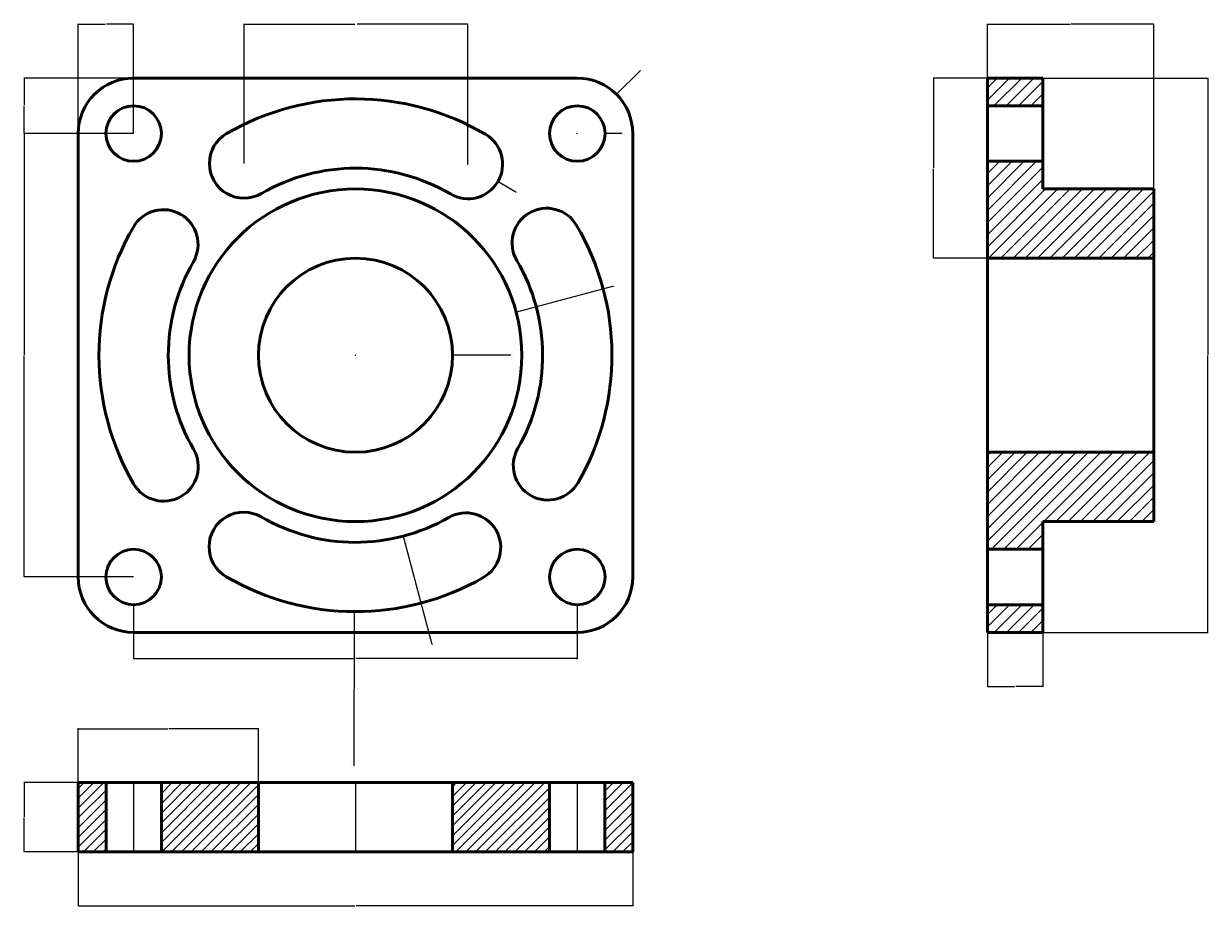
# Model space of a CAD drawing. Units: inches. Extents: x 17 to 444, y -186 to 133.
import ezdxf

# ---------------------------------------------------------------- set-up
doc = ezdxf.new("R2010")
doc.units = ezdxf.units.IN
doc.header["$MEASUREMENT"] = 0
doc.linetypes.add('CENTER', pattern=[50.8, 31.75, -6.35, 6.35, -6.35])
for name, color, linetype, lineweight in [('M-CNTR', 4, 'CENTER', 18), ('M-DIMS', 2, 'Continuous', 18), ('M-HATC', 8, 'Continuous', 18), ('M-OUTL', 7, 'Continuous', 50)]:
    doc.layers.add(name, color=color, linetype=linetype, lineweight=lineweight)
doc.styles.get("Standard").update_dxf_attribs({"font": 'arial.ttf'})
doc.dimstyles.get("Standard").update_dxf_attribs({"dimtxt": 0.18, "dimasz": 0.18, "dimexe": 0.18, "dimexo": 0.0625, "dimgap": 0.09, "dimtad": 0, "dimtih": 1, "dimtoh": 1, "dimdec": 4, "dimzin": 0, "dimdsep": 46, "dimtxsty": 'Standard', "dimcen": 0.09, "dimadec": 0, "dimazin": 0, "dimtfac": 1, "dimtdec": 4, "dimtofl": 0, "dimtmove": 0, "dimatfit": 3, "dimfxl": 1, "dimtolj": 1, "dimtzin": 0, "dimarcsym": 0})
pattern_1 = [(45, (-581.398, -124.7495), (-2.209709, 2.209709), [])]
pattern_2 = [(45, (-581.398, -124.7495), (-1.767767, 1.767767), [])]

# ---------------------------------------------------------------- blocks, each defined once
blk = doc.blocks.new('FLANGE-MOUNT-HOLE-D20')
blk.add_circle((10, 10), 10)
blk = doc.blocks.new('*D2')
at = {"layer": 'Defpoints', "color": 0, "transparency": 16777216}
for p in [(36.63, -165.99), (236.63, -165.99), (236.63, -185.44)]:
    blk.add_point(p, dxfattribs=at)
at = {"layer": 'M-DIMS', "color": 0, "lineweight": -2, "transparency": 16777216}
for p, q in [((36.63, -166.06), (36.63, -185.62)), ((236.63, -166.06), (236.63, -185.62)), ((36.81, -185.44), (136.34, -185.44)), ((236.45, -185.44), (136.92, -185.44))]:
    blk.add_line(p, q, dxfattribs=at)
at = {"layer": 'M-DIMS', "color": 0, "transparency": 16777216}
for points in [[(36.81, -185.41), (36.81, -185.47), (36.63, -185.44)], [(236.45, -185.41), (236.45, -185.47), (236.63, -185.44)]]:
    blk.add_solid(points, dxfattribs=at)
at = {"layer": 'M-DIMS', "color": 0, "transparency": 16777216, "insert": (136.63, -185.44), "char_height": 0.18, "attachment_point": 5}
blk.add_mtext('\\A1;200', dxfattribs=at)
blk = doc.blocks.new('*D3')
at = {"layer": 'Defpoints', "color": 0, "transparency": 16777216}
for p in [(384.54, 113.19), (443.99, 113.19), (384.54, -86.81)]:
    blk.add_point(p, dxfattribs=at)
at = {"layer": 'M-DIMS', "color": 0, "lineweight": -2, "transparency": 16777216}
for p, q in [((384.6, 113.19), (444.17, 113.19)), ((443.99, 113.01), (443.99, 13.37)), ((443.99, -86.63), (443.99, 13.01)), ((384.6, -86.81), (444.17, -86.81))]:
    blk.add_line(p, q, dxfattribs=at)
at = {"layer": 'M-DIMS', "color": 0, "transparency": 16777216}
for points in [[(443.96, 113.01), (444.02, 113.01), (443.99, 113.19)], [(443.96, -86.63), (444.02, -86.63), (443.99, -86.81)]]:
    blk.add_solid(points, dxfattribs=at)
at = {"layer": 'M-DIMS', "color": 0, "transparency": 16777216, "insert": (443.99, 13.19), "char_height": 0.18, "attachment_point": 5}
blk.add_mtext('\\A1;200', dxfattribs=at)
blk = doc.blocks.new('*D4')
at = {"layer": 'Defpoints', "color": 0, "transparency": 16777216}
for p in [(56.63, -76.81), (216.63, -76.81), (56.63, -96.26)]:
    blk.add_point(p, dxfattribs=at)
at = {"layer": 'M-DIMS', "color": 0, "lineweight": -2, "transparency": 16777216}
for p, q in [((56.63, -76.87), (56.63, -96.44)), ((216.63, -76.87), (216.63, -96.44)), ((56.81, -96.26), (136.35, -96.26)), ((216.45, -96.26), (136.91, -96.26))]:
    blk.add_line(p, q, dxfattribs=at)
at = {"layer": 'M-DIMS', "color": 0, "transparency": 16777216}
for points in [[(56.81, -96.23), (56.81, -96.29), (56.63, -96.26)], [(216.45, -96.23), (216.45, -96.29), (216.63, -96.26)]]:
    blk.add_solid(points, dxfattribs=at)
at = {"layer": 'M-DIMS', "color": 0, "transparency": 16777216, "insert": (136.63, -96.26), "char_height": 0.18, "attachment_point": 5}
blk.add_mtext('\\A1;160', dxfattribs=at)
blk = doc.blocks.new('*D5')
at = {"layer": 'Defpoints', "color": 0, "transparency": 16777216}
for p in [(17.18, 93.19), (56.63, 93.19), (56.63, -66.81)]:
    blk.add_point(p, dxfattribs=at)
at = {"layer": 'M-DIMS', "color": 0, "lineweight": -2, "transparency": 16777216}
for p, q in [((56.56, 93.19), (17, 93.19)), ((17.18, 93.01), (17.18, 13.37)), ((17.18, -66.63), (17.18, 13.01)), ((56.56, -66.81), (17, -66.81))]:
    blk.add_line(p, q, dxfattribs=at)
at = {"layer": 'M-DIMS', "color": 0, "transparency": 16777216}
for points in [[(17.15, 93.01), (17.21, 93.01), (17.18, 93.19)], [(17.15, -66.63), (17.21, -66.63), (17.18, -66.81)]]:
    blk.add_solid(points, dxfattribs=at)
at = {"layer": 'M-DIMS', "color": 0, "transparency": 16777216, "insert": (17.18, 13.19), "char_height": 0.18, "attachment_point": 5}
blk.add_mtext('\\A1;160', dxfattribs=at)
blk = doc.blocks.new('*D6')
at = {"layer": 'Defpoints', "color": 0, "transparency": 16777216}
for p in [(56.63, 132.64), (36.63, 93.19), (56.63, 93.19)]:
    blk.add_point(p, dxfattribs=at)
at = {"layer": 'M-DIMS', "color": 0, "lineweight": -2, "transparency": 16777216}
for p, q in [((36.63, 93.25), (36.63, 132.82)), ((36.81, 132.64), (46.41, 132.64)), ((56.45, 132.64), (46.85, 132.64)), ((56.63, 93.25), (56.63, 132.82))]:
    blk.add_line(p, q, dxfattribs=at)
at = {"layer": 'M-DIMS', "color": 0, "transparency": 16777216}
for points in [[(36.81, 132.67), (36.81, 132.61), (36.63, 132.64)], [(56.45, 132.67), (56.45, 132.61), (56.63, 132.64)]]:
    blk.add_solid(points, dxfattribs=at)
at = {"layer": 'M-DIMS', "color": 0, "transparency": 16777216, "insert": (46.63, 132.64), "char_height": 0.18, "attachment_point": 5}
blk.add_mtext('\\A1;20', dxfattribs=at)
blk = doc.blocks.new('*D7')
at = {"layer": 'Defpoints', "color": 0, "transparency": 16777216}
for p in [(17.18, 113.19), (56.63, 113.19), (56.63, 93.19)]:
    blk.add_point(p, dxfattribs=at)
at = {"layer": 'M-DIMS', "color": 0, "lineweight": -2, "transparency": 16777216}
for p, q in [((56.56, 113.19), (17, 113.19)), ((17.18, 113.01), (17.18, 103.37)), ((17.18, 93.37), (17.18, 103.01)), ((56.56, 93.19), (17, 93.19))]:
    blk.add_line(p, q, dxfattribs=at)
at = {"layer": 'M-DIMS', "color": 0, "transparency": 16777216}
for points in [[(17.15, 113.01), (17.21, 113.01), (17.18, 113.19)], [(17.15, 93.37), (17.21, 93.37), (17.18, 93.19)]]:
    blk.add_solid(points, dxfattribs=at)
at = {"layer": 'M-DIMS', "color": 0, "transparency": 16777216, "insert": (17.18, 103.19), "char_height": 0.18, "attachment_point": 5}
blk.add_mtext('\\A1;20', dxfattribs=at)
blk = doc.blocks.new('*D8')
at = {"layer": 'Defpoints', "color": 0, "transparency": 16777216}
for p in [(177.18, 132.64), (96.44, 82.37), (177.18, 82.15)]:
    blk.add_point(p, dxfattribs=at)
at = {"layer": 'M-DIMS', "color": 0, "lineweight": -2, "transparency": 16777216}
for p, q in [((96.44, 82.43), (96.44, 132.82)), ((96.62, 132.64), (136.42, 132.64)), ((177, 132.64), (137.21, 132.64)), ((177.18, 82.21), (177.18, 132.82))]:
    blk.add_line(p, q, dxfattribs=at)
at = {"layer": 'M-DIMS', "color": 0, "transparency": 16777216}
for points in [[(96.62, 132.67), (96.62, 132.61), (96.44, 132.64)], [(177, 132.67), (177, 132.61), (177.18, 132.64)]]:
    blk.add_solid(points, dxfattribs=at)
at = {"layer": 'M-DIMS', "color": 0, "transparency": 16777216, "insert": (136.81, 132.64), "char_height": 0.18, "attachment_point": 5}
blk.add_mtext('\\A1;80.74', dxfattribs=at)
blk = doc.blocks.new('*D9')
at = {"layer": 'Defpoints', "color": 0, "transparency": 16777216}
for p in [(364.54, -86.81), (384.54, -86.81), (364.54, -106.26)]:
    blk.add_point(p, dxfattribs=at)
at = {"layer": 'M-DIMS', "color": 0, "lineweight": -2, "transparency": 16777216}
for p, q in [((364.54, -86.87), (364.54, -106.44)), ((384.54, -86.87), (384.54, -106.44)), ((364.72, -106.26), (374.32, -106.26)), ((384.36, -106.26), (374.76, -106.26))]:
    blk.add_line(p, q, dxfattribs=at)
at = {"layer": 'M-DIMS', "color": 0, "transparency": 16777216}
for points in [[(364.72, -106.23), (364.72, -106.29), (364.54, -106.26)], [(384.36, -106.23), (384.36, -106.29), (384.54, -106.26)]]:
    blk.add_solid(points, dxfattribs=at)
at = {"layer": 'M-DIMS', "color": 0, "transparency": 16777216, "insert": (374.54, -106.26), "char_height": 0.18, "attachment_point": 5}
blk.add_mtext('\\A1;20', dxfattribs=at)
blk = doc.blocks.new('*D10')
at = {"layer": 'Defpoints', "color": 0, "transparency": 16777216}
for p in [(424.54, 132.64), (364.54, 113.19), (424.54, 73.19)]:
    blk.add_point(p, dxfattribs=at)
at = {"layer": 'M-DIMS', "color": 0, "lineweight": -2, "transparency": 16777216}
for p, q in [((364.54, 113.25), (364.54, 132.82)), ((364.72, 132.64), (394.32, 132.64)), ((424.36, 132.64), (394.76, 132.64)), ((424.54, 73.25), (424.54, 132.82))]:
    blk.add_line(p, q, dxfattribs=at)
at = {"layer": 'M-DIMS', "color": 0, "transparency": 16777216}
for points in [[(364.72, 132.67), (364.72, 132.61), (364.54, 132.64)], [(424.36, 132.67), (424.36, 132.61), (424.54, 132.64)]]:
    blk.add_solid(points, dxfattribs=at)
at = {"layer": 'M-DIMS', "color": 0, "transparency": 16777216, "insert": (394.54, 132.64), "char_height": 0.18, "attachment_point": 5}
blk.add_mtext('\\A1;60', dxfattribs=at)
blk = doc.blocks.new('*D11')
at = {"layer": 'Defpoints', "color": 0, "transparency": 16777216}
for p in [(17.18, -140.99), (36.63, -140.99), (36.63, -165.99)]:
    blk.add_point(p, dxfattribs=at)
at = {"layer": 'M-DIMS', "color": 0, "lineweight": -2, "transparency": 16777216}
for p, q in [((36.56, -140.99), (17, -140.99)), ((17.18, -141.17), (17.18, -153.31)), ((17.18, -165.81), (17.18, -153.68)), ((36.56, -165.99), (17, -165.99))]:
    blk.add_line(p, q, dxfattribs=at)
at = {"layer": 'M-DIMS', "color": 0, "transparency": 16777216}
for points in [[(17.15, -141.17), (17.21, -141.17), (17.18, -140.99)], [(17.15, -165.81), (17.21, -165.81), (17.18, -165.99)]]:
    blk.add_solid(points, dxfattribs=at)
at = {"layer": 'M-DIMS', "color": 0, "transparency": 16777216, "insert": (17.18, -153.49), "char_height": 0.18, "attachment_point": 5}
blk.add_mtext('\\A1;25', dxfattribs=at)
blk = doc.blocks.new('*D12')
at = {"layer": 'Defpoints', "color": 0, "transparency": 16777216}
for p in [(101.63, -121.54), (36.63, -140.99), (101.63, -140.99)]:
    blk.add_point(p, dxfattribs=at)
at = {"layer": 'M-DIMS', "color": 0, "lineweight": -2, "transparency": 16777216}
for p, q in [((36.63, -140.93), (36.63, -121.36)), ((36.81, -121.54), (68.91, -121.54)), ((101.45, -121.54), (69.35, -121.54)), ((101.63, -140.93), (101.63, -121.36))]:
    blk.add_line(p, q, dxfattribs=at)
at = {"layer": 'M-DIMS', "color": 0, "transparency": 16777216}
for points in [[(36.81, -121.51), (36.81, -121.57), (36.63, -121.54)], [(101.45, -121.51), (101.45, -121.57), (101.63, -121.54)]]:
    blk.add_solid(points, dxfattribs=at)
at = {"layer": 'M-DIMS', "color": 0, "transparency": 16777216, "insert": (69.13, -121.54), "char_height": 0.18, "attachment_point": 5}
blk.add_mtext('\\A1;65', dxfattribs=at)
blk = doc.blocks.new('*D13')
at = {"layer": 'Defpoints', "color": 0, "transparency": 16777216}
for p in [(345.09, 113.19), (364.54, 113.19), (364.54, 48.19)]:
    blk.add_point(p, dxfattribs=at)
at = {"layer": 'M-DIMS', "color": 0, "lineweight": -2, "transparency": 16777216}
for p, q in [((364.48, 113.19), (344.91, 113.19)), ((345.09, 113.01), (345.09, 80.87)), ((345.09, 48.37), (345.09, 80.51)), ((364.48, 48.19), (344.91, 48.19))]:
    blk.add_line(p, q, dxfattribs=at)
at = {"layer": 'M-DIMS', "color": 0, "transparency": 16777216}
for points in [[(345.06, 113.01), (345.12, 113.01), (345.09, 113.19)], [(345.06, 48.37), (345.12, 48.37), (345.09, 48.19)]]:
    blk.add_solid(points, dxfattribs=at)
at = {"layer": 'M-DIMS', "color": 0, "transparency": 16777216, "insert": (345.09, 80.69), "char_height": 0.18, "attachment_point": 5}
blk.add_mtext('\\A1;65', dxfattribs=at)
blk = doc.blocks.new('*D14')
at = {"layer": 'Defpoints', "color": 0, "transparency": 16777216}
for p in [(206.63, 93.19), (226.63, 93.19)]:
    blk.add_point(p, dxfattribs=at)
at = {"layer": 'M-DIMS', "color": 0, "lineweight": -2, "transparency": 16777216}
for p, q in [((216.54, 93.19), (216.72, 93.19)), ((216.63, 93.1), (216.63, 93.28)), ((232.63, 93.19), (226.81, 93.19))]:
    blk.add_line(p, q, dxfattribs=at)
at = {"layer": 'M-DIMS', "color": 0, "transparency": 16777216}
blk.add_solid([(226.81, 93.22), (226.81, 93.16), (226.63, 93.19)], dxfattribs=at)
at = {"layer": 'M-DIMS', "color": 0, "transparency": 16777216, "insert": (233.13, 93.19), "char_height": 0.18, "attachment_point": 5}
blk.add_mtext('\\A1;4X ∅20', dxfattribs=at)
blk = doc.blocks.new('*D15')
at = {"layer": 'Defpoints', "color": 0, "transparency": 16777216}
for p in [(230.77, 107.33), (216.63, 93.19)]:
    blk.add_point(p, dxfattribs=at)
at = {"layer": 'M-DIMS', "color": 0, "lineweight": -2, "transparency": 16777216}
for p, q in [((239.25, 115.82), (230.89, 107.46)), ((239.43, 115.82), (239.25, 115.82)), ((216.54, 93.19), (216.72, 93.19)), ((216.63, 93.1), (216.63, 93.28))]:
    blk.add_line(p, q, dxfattribs=at)
at = {"layer": 'M-DIMS', "color": 0, "transparency": 16777216}
blk.add_solid([(230.87, 107.48), (230.92, 107.44), (230.77, 107.33)], dxfattribs=at)
at = {"layer": 'M-DIMS', "color": 0, "transparency": 16777216, "insert": (239.93, 115.82), "char_height": 0.18, "attachment_point": 5}
blk.add_mtext('\\A1;4X R20', dxfattribs=at)
blk = doc.blocks.new('*D16')
at = {"layer": 'Defpoints', "color": 0, "transparency": 16777216}
for p in [(101.63, 13.19), (171.63, 13.19)]:
    blk.add_point(p, dxfattribs=at)
at = {"layer": 'M-DIMS', "color": 0, "lineweight": -2, "transparency": 16777216}
for p, q in [((136.54, 13.19), (136.72, 13.19)), ((136.63, 13.1), (136.63, 13.28)), ((192.63, 13.19), (171.81, 13.19))]:
    blk.add_line(p, q, dxfattribs=at)
at = {"layer": 'M-DIMS', "color": 0, "transparency": 16777216}
blk.add_solid([(171.81, 13.22), (171.81, 13.16), (171.63, 13.19)], dxfattribs=at)
at = {"layer": 'M-DIMS', "color": 0, "transparency": 16777216, "insert": (192.94, 13.19), "char_height": 0.18, "attachment_point": 5}
blk.add_mtext('\\A1;∅70', dxfattribs=at)
blk = doc.blocks.new('*D17')
at = {"layer": 'Defpoints', "color": 0, "transparency": 16777216}
for p in [(194.58, 28.72), (78.67, -2.34)]:
    blk.add_point(p, dxfattribs=at)
at = {"layer": 'M-DIMS', "color": 0, "lineweight": -2, "transparency": 16777216}
for p, q in [((229.35, 38.04), (194.75, 28.77)), ((229.53, 38.04), (229.35, 38.04)), ((136.54, 13.19), (136.72, 13.19)), ((136.63, 13.1), (136.63, 13.28))]:
    blk.add_line(p, q, dxfattribs=at)
at = {"layer": 'M-DIMS', "color": 0, "transparency": 16777216}
blk.add_solid([(194.75, 28.8), (194.76, 28.74), (194.58, 28.72)], dxfattribs=at)
at = {"layer": 'M-DIMS', "color": 0, "transparency": 16777216, "insert": (229.92, 38.04), "char_height": 0.18, "attachment_point": 5}
blk.add_mtext('\\A1;∅120', dxfattribs=at)
blk = doc.blocks.new('*D18')
at = {"layer": 'Defpoints', "color": 0, "transparency": 16777216}
for p in [(136.63, 13.19), (136.33, -79.31)]:
    blk.add_point(p, dxfattribs=at)
at = {"layer": 'M-DIMS', "color": 0, "lineweight": -2, "transparency": 16777216}
for p, q in [((136.54, 13.19), (136.72, 13.19)), ((136.63, 13.1), (136.63, 13.28)), ((136.16, -134.81), (136.33, -79.49)), ((135.98, -134.81), (136.16, -134.81))]:
    blk.add_line(p, q, dxfattribs=at)
at = {"layer": 'M-DIMS', "color": 0, "transparency": 16777216}
blk.add_solid([(136.3, -79.49), (136.36, -79.49), (136.33, -79.31)], dxfattribs=at)
at = {"layer": 'M-DIMS', "color": 0, "transparency": 16777216, "insert": (135.37, -134.81), "char_height": 0.18, "attachment_point": 5}
blk.add_mtext('\\A1;4X R92.5', dxfattribs=at)
blk = doc.blocks.new('*D19')
at = {"layer": 'Defpoints', "color": 0, "transparency": 16777216}
for p in [(136.63, 13.19), (153.88, -52.07)]:
    blk.add_point(p, dxfattribs=at)
at = {"layer": 'M-DIMS', "color": 0, "lineweight": -2, "transparency": 16777216}
for p, q in [((136.54, 13.19), (136.72, 13.19)), ((136.63, 13.1), (136.63, 13.28)), ((164.24, -91.22), (153.93, -52.24)), ((164.42, -91.22), (164.24, -91.22))]:
    blk.add_line(p, q, dxfattribs=at)
at = {"layer": 'M-DIMS', "color": 0, "transparency": 16777216}
blk.add_solid([(153.96, -52.23), (153.9, -52.25), (153.88, -52.07)], dxfattribs=at)
at = {"layer": 'M-DIMS', "color": 0, "transparency": 16777216, "insert": (165.02, -91.22), "char_height": 0.18, "attachment_point": 5}
blk.add_mtext('\\A1;4X R67.5', dxfattribs=at)
blk = doc.blocks.new('*D20')
at = {"layer": 'Defpoints', "color": 0, "transparency": 16777216}
for p in [(177.18, 82.15), (187.96, 75.81)]:
    blk.add_point(p, dxfattribs=at)
at = {"layer": 'M-DIMS', "color": 0, "lineweight": -2, "transparency": 16777216}
for p, q in [((177.09, 82.15), (177.27, 82.15)), ((177.18, 82.06), (177.18, 82.24)), ((194.42, 72.01), (188.11, 75.72)), ((194.6, 72.01), (194.42, 72.01))]:
    blk.add_line(p, q, dxfattribs=at)
at = {"layer": 'M-DIMS', "color": 0, "transparency": 16777216}
blk.add_solid([(188.13, 75.75), (188.1, 75.69), (187.96, 75.81)], dxfattribs=at)
at = {"layer": 'M-DIMS', "color": 0, "transparency": 16777216, "insert": (195.21, 72.01), "char_height": 0.18, "attachment_point": 5}
blk.add_mtext('\\A1;8X R12.5', dxfattribs=at)

msp = doc.modelspace()

# ---------------------------------------------------------------- hatches: boundary and pattern name
at = {"layer": 'M-HATC'}
h = msp.add_hatch(dxfattribs=at)
h.set_pattern_fill('ANSI31', color=256, scale=25)
h.set_pattern_definition(pattern_1)
h.paths.add_polyline_path([(384.541, 113.19), (364.541, 113.19), (364.541, 103.19), (384.541, 103.19)])
h.paths.add_polyline_path([(424.541, 73.19), (384.541, 73.19), (384.541, 83.19), (364.541, 83.19), (364.541, 48.19), (424.541, 48.19)])
h = msp.add_hatch(dxfattribs=at)
h.set_pattern_fill('ANSI31', color=256, scale=25)
h.set_pattern_definition(pattern_1)
h.paths.add_polyline_path([(364.541, -76.81), (364.541, -86.81), (384.541, -86.81), (384.541, -76.81)])
h.paths.add_polyline_path([(364.541, -21.81), (364.541, -56.81), (384.541, -56.81), (384.541, -46.81), (424.541, -46.81), (424.541, -21.81)])
h = msp.add_hatch(dxfattribs=at)
h.set_pattern_fill('ANSI31', color=256, scale=20)
h.set_pattern_definition(pattern_2)
h.paths.add_polyline_path([(46.676, -140.995), (36.626, -140.995), (36.626, -165.995), (46.676, -165.995)])
h.paths.add_polyline_path([(101.626, -140.995), (66.626, -140.995), (66.626, -165.995), (101.626, -165.995)])
h = msp.add_hatch(dxfattribs=at)
h.set_pattern_fill('ANSI31', color=256, scale=20)
h.set_pattern_definition(pattern_2)
h.paths.add_polyline_path([(236.626, -140.995), (226.576, -140.995), (226.576, -165.995), (236.626, -165.995)])
h.paths.add_polyline_path([(171.626, -140.995), (171.626, -165.995), (206.626, -165.995), (206.626, -140.995)])

# ---------------------------------------------------------------- linework, layer by layer
at = {"layer": 'M-CNTR'}
for p, q in [((56.626, -140.995), (56.626, -165.995)), ((136.626, -140.995), (136.626, -165.995)), ((216.626, -140.995), (216.626, -165.995))]:
    msp.add_line(p, q, dxfattribs=at)
at = {"layer": 'M-OUTL'}
for p, q in [((216.626, 113.19), (56.626, 113.19)), ((384.541, 113.19), (364.541, 113.19)), ((364.541, 113.19), (364.541, 48.19)), ((384.541, 73.19), (384.541, 113.19)), ((364.541, 103.19), (384.541, 103.19)), ((36.626, 93.19), (36.626, -66.81)), ((236.626, 13.19), (236.626, 93.19)), ((364.541, 83.19), (384.541, 83.19)), ((424.541, 73.19), (384.541, 73.19)), ((424.541, 48.19), (424.541, 73.19)), ((364.541, 13.19), (364.541, 48.19)), ((364.541, 48.19), (424.541, 48.19)), ((424.541, 48.19), (424.541, 13.19)), ((236.626, -66.81), (236.626, 13.19)), ((364.541, 13.19), (364.541, -21.81)), ((424.541, -21.81), (424.541, 13.19)), ((364.541, -21.81), (424.541, -21.81)), ((364.541, -86.81), (364.541, -21.81)), ((424.541, -21.81), (424.541, -46.81)), ((424.541, -46.81), (384.541, -46.81)), ((384.541, -46.81), (384.541, -86.81)), ((364.541, -56.81), (384.541, -56.81)), ((364.541, -76.81), (384.541, -76.81)), ((56.626, -86.81), (216.626, -86.81)), ((384.541, -86.81), (364.541, -86.81)), ((36.626, -140.995), (136.626, -140.995)), ((36.626, -140.995), (36.626, -165.995)), ((46.676, -165.995), (46.676, -140.995)), ((46.676, -140.995), (56.626, -140.995)), ((66.626, -165.995), (66.626, -140.995)), ((66.626, -140.995), (101.626, -140.995)), ((101.626, -140.995), (101.626, -165.995)), ((236.626, -140.995), (136.626, -140.995)), ((206.626, -140.995), (171.626, -140.995)), ((171.626, -140.995), (171.626, -165.995)), ((206.626, -165.995), (206.626, -140.995)), ((226.576, -140.995), (216.626, -140.995)), ((226.576, -165.995), (226.576, -140.995)), ((236.626, -140.995), (236.626, -165.995)), ((136.626, -165.995), (36.626, -165.995)), ((36.626, -165.995), (46.676, -165.995)), ((56.626, -165.995), (66.626, -165.995)), ((136.626, -165.995), (236.626, -165.995)), ((216.626, -165.995), (206.626, -165.995)), ((236.626, -165.995), (226.576, -165.995))]:
    msp.add_line(p, q, dxfattribs=at)
for radius in [60, 35]:
    msp.add_circle((136.626, 13.19), radius, dxfattribs=at)
for centre, radius, start, end in [((56.626, 93.19), 20, 90, 180), ((216.626, 93.19), 20, 0, 90), ((136.626, 13.19), 92.5, 59.53857, 120.14971), ((96.445, 82.368), 12.5, 120.14971, 300.14971), ((177.182, 82.148), 12.5, 239.53857, 59.53857), ((136.626, 13.19), 67.5, 59.53857, 120.14971), ((67.353, 53.208), 12.5, 329.98591, 149.98591), ((205.597, 53.724), 12.5, 30.44259, 210.44259), ((136.626, 13.19), 92.5, 330.21038, 30.44259), ((136.626, 13.19), 92.5, 149.98591, 210.11469), ((136.626, 13.19), 67.5, 330.21038, 30.44259), ((136.626, 13.19), 67.5, 149.98591, 210.11469), ((67.424, -26.948), 12.5, 210.11469, 30.11469), ((206.054, -26.555), 12.5, 150.21038, 330.21038), ((96.324, -55.917), 12.5, 59.75029, 239.75029), ((136.626, 13.19), 67.5, 239.75029, 299.88965), ((176.492, -56.168), 12.5, 299.88965, 119.88965), ((56.626, -66.81), 20, 180, 270), ((136.626, 13.19), 92.5, 239.75029, 299.88965), ((216.626, -66.81), 20, 270, 0)]:
    msp.add_arc(centre, radius, start, end, dxfattribs=at)

# ---------------------------------------------------------------- block references
for p in [(46.626, 83.19), (206.626, 83.19), (46.626, -76.81), (206.626, -76.81)]:
    msp.add_blockref('FLANGE-MOUNT-HOLE-D20', p, dxfattribs=at)

# ---------------------------------------------------------------- dimensions: what is measured, and where the dimension line sits
at = {"layer": 'M-DIMS'}
for base, p1, p2, override, picture, middle in [((56.626, 132.64), (36.626, 93.19), (56.626, 93.19), {"dimdec": 0, "dimlfac": 1, "dimrnd": 0, "dimzin": 0, "dimdsep": 46, "dimlunit": 2}, '*D6', (46.626, 132.64)), ((177.182, 132.64), (96.445, 82.368), (177.182, 82.148), {"dimdec": 2, "dimlfac": 1, "dimrnd": 0, "dimzin": 0, "dimdsep": 46, "dimlunit": 2}, '*D8', (136.814, 132.64)), ((424.541, 132.64), (364.541, 113.19), (424.541, 73.19), {"dimdec": 0, "dimlfac": 1, "dimrnd": 0, "dimzin": 0, "dimdsep": 46, "dimlunit": 2}, '*D10', (394.541, 132.64)), ((101.626, -121.545), (36.626, -140.995), (101.626, -140.995), {"dimdec": 0, "dimlfac": 1, "dimrnd": 0, "dimzin": 0, "dimdsep": 46, "dimlunit": 2}, '*D12', (69.126, -121.545)), ((236.626, -185.445), (36.626, -165.995), (236.626, -165.995), {"dimdec": 0, "dimlfac": 1, "dimrnd": 0, "dimzin": 0, "dimdsep": 46, "dimlunit": 2}, '*D2', (136.626, -185.445))]:
    dim = msp.add_linear_dim(base=base, p1=p1, p2=p2, dimstyle='Standard', override=override, dxfattribs=at)
    dim.commit()
    dim.dimension.update_dxf_attribs({"geometry": picture, "text_midpoint": middle})
for center, mpoint, text, override, picture, middle in [((216.626, 93.19), (230.768, 107.333), '4X <>', {"dimdec": 0, "dimlfac": 1, "dimrnd": 0, "dimzin": 0, "dimdsep": 46, "dimlunit": 2}, '*D15', (239.935, 115.818)), ((177.182, 82.148), (187.957, 75.811), '8X <>', {"dimdec": 1, "dimlfac": 1, "dimrnd": 0, "dimzin": 0, "dimdsep": 46, "dimlunit": 2}, '*D20', (195.206, 72.009)), ((136.626, 13.19), (136.335, -79.309), '4X <>', {"dimdec": 1, "dimlfac": 1, "dimrnd": 0, "dimzin": 0, "dimdsep": 46, "dimlunit": 2}, '*D18', (135.373, -134.809)), ((136.626, 13.19), (153.882, -52.067), '4X <>', {"dimdec": 1, "dimlfac": 1, "dimrnd": 0, "dimzin": 0, "dimdsep": 46, "dimlunit": 2}, '*D19', (165.023, -91.221))]:
    dim = msp.add_radius_dim(center=center, mpoint=mpoint, text=text, dimstyle='Standard', override=override, dxfattribs=at)
    dim.commit()
    dim.dimension.update_dxf_attribs({"geometry": picture, "text_midpoint": middle, "dimtype": 164})
for base, p1, p2, angle, picture, middle in [((17.176, 113.19), (56.626, 93.19), (56.626, 113.19), 90, '*D7', (17.176, 103.19)), ((345.091, 113.19), (364.541, 48.19), (364.541, 113.19), 90, '*D13', (345.091, 80.69)), ((443.991, 113.19), (384.541, -86.81), (384.541, 113.19), 90, '*D3', (443.991, 13.19)), ((17.176, 93.19), (56.626, -66.81), (56.626, 93.19), 90, '*D5', (17.176, 13.19)), ((56.626, -96.26), (216.626, -76.81), (56.626, -76.81), 180, '*D4', (136.626, -96.26)), ((364.541, -106.26), (384.541, -86.81), (364.541, -86.81), 180, '*D9', (374.541, -106.26)), ((17.176, -140.995), (36.626, -165.995), (36.626, -140.995), 90, '*D11', (17.176, -153.495))]:
    dim = msp.add_linear_dim(base=base, p1=p1, p2=p2, angle=angle, dimstyle='Standard', override={"dimdec": 0, "dimlfac": 1, "dimrnd": 0, "dimzin": 0, "dimdsep": 46, "dimlunit": 2}, dxfattribs=at)
    dim.commit()
    dim.dimension.update_dxf_attribs({"geometry": picture, "text_midpoint": middle})
dim = msp.add_diameter_dim_2p(p1=(206.626, 93.191), p2=(226.626, 93.19), text='4X <>', dimstyle='Standard', override={"dimdec": 0, "dimlfac": 1, "dimrnd": 0, "dimzin": 0, "dimdsep": 46, "dimlunit": 2}, dxfattribs=at)
dim.commit()
dim.dimension.update_dxf_attribs({"geometry": '*D14', "text_midpoint": (232.626, 93.19), "dimtype": 163})
for p1, p2, picture, middle in [((78.67, -2.339), (194.581, 28.72), '*D17', (229.921, 38.038)), ((101.626, 13.191), (171.626, 13.19), '*D16', (192.626, 13.19))]:
    dim = msp.add_diameter_dim_2p(p1=p1, p2=p2, dimstyle='Standard', override={"dimdec": 0, "dimlfac": 1, "dimrnd": 0, "dimzin": 0, "dimdsep": 46, "dimlunit": 2}, dxfattribs=at)
    dim.commit()
    dim.dimension.update_dxf_attribs({"geometry": picture, "text_midpoint": middle, "dimtype": 163})

doc.saveas('drawing.dxf')
